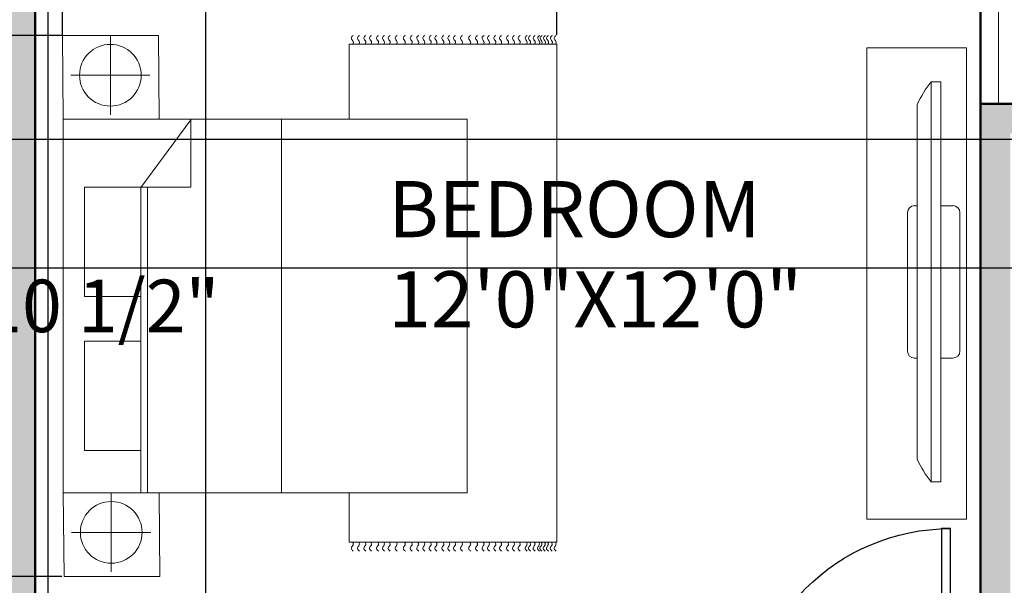
# Model space of a CAD drawing. Units: inches. Extents: x 22042254 to 25404563, y 17568978 to 17626777.
# Tile 40 of 45: x 22179790 to 22179940, y 17626607 to 17626694. Entities that reach past the tile are written whole.
import ezdxf

# ---------------------------------------------------------------- set-up
doc = ezdxf.new("R2010")
doc.units = ezdxf.units.IN
doc.header["$MEASUREMENT"] = 0
for name, color, linetype, lineweight in [('A-ANNO-DIMS', 2, 'Continuous', 18), ('A-AREA-IDEN', 7, 'Continuous', 18), ('A-FLOR-OPEN', 252, 'Continuous', 18), ('A-WALL-PATT', 244, 'Continuous', 13), ('doors', 4, 'Continuous', 25), ('furniture', 8, 'Continuous', 18), ('walls', 252, 'Continuous', 50)]:
    doc.layers.add(name, color=color, linetype=linetype, lineweight=lineweight)
doc.styles.get("Standard").update_dxf_attribs({"font": 'arial.ttf'})
doc.dimstyles.get("Standard").update_dxf_attribs({"dimtxt": 8, "dimasz": 0.18, "dimexe": 0.18, "dimexo": 0.0625, "dimgap": 0.09, "dimtad": 0, "dimtih": 1, "dimtoh": 1, "dimzin": 0, "dimdsep": 46, "dimlunit": 3, "dimtxsty": 'Standard', "dimcen": 0.09, "dimadec": 0, "dimazin": 0, "dimtfac": 1, "dimtofl": 0, "dimtmove": 0, "dimatfit": 3, "dimfxl": 1, "dimtolj": 1, "dimtzin": 0, "dimarcsym": 0})

# ---------------------------------------------------------------- blocks, each defined once
blk = doc.blocks.new('CARPET')
at = {"layer": 'furniture'}
for p, q in [((-51.53, -98.11), (-51.53, -55.12)), ((-51.53, -55.12), (-41.27, -55.12)), ((36, -55.12), (51.55, -55.12)), ((51.55, -55.12), (51.55, -98.11)), ((51.55, -98.11), (-51.53, -98.11))]:
    blk.add_line(p, q, dxfattribs=at)
for points, knots in [([(-53.37, -55.99), (-53.22, -55.8), (-52.9, -55.41), (-52.34, -55.8), (-51.89, -56.08), (-51.65, -55.91), (-51.53, -55.83)], [0, 0, 0, 0, 0.653278, 1.290138, 1.740457, 2.114451, 2.114451, 2.114451, 2.114451]), ([(-53.37, -57.26), (-53.22, -57.07), (-52.9, -56.67), (-52.34, -57.07), (-51.89, -57.35), (-51.65, -57.17), (-51.53, -57.1)], [0, 0, 0, 0, 0.653278, 1.290138, 1.740457, 2.114451, 2.114451, 2.114451, 2.114451]), ([(53.37, -55.99), (53.22, -55.8), (52.9, -55.41), (52.34, -55.8), (51.89, -56.08), (51.65, -55.91), (51.53, -55.83)], [0, 0, 0, 0, 0.653278, 1.290138, 1.740457, 2.114451, 2.114451, 2.114451, 2.114451]), ([(53.37, -57.26), (53.22, -57.07), (52.9, -56.67), (52.34, -57.07), (51.89, -57.35), (51.65, -57.17), (51.53, -57.1)], [0, 0, 0, 0, 0.653278, 1.290138, 1.740457, 2.114451, 2.114451, 2.114451, 2.114451]), ([(-53.37, -58.59), (-53.22, -58.4), (-52.9, -58.01), (-52.34, -58.4), (-51.89, -58.68), (-51.65, -58.5), (-51.53, -58.43)], [0, 0, 0, 0, 0.653278, 1.290138, 1.740457, 2.114451, 2.114451, 2.114451, 2.114451]), ([(53.37, -58.59), (53.22, -58.4), (52.9, -58.01), (52.34, -58.4), (51.89, -58.68), (51.65, -58.5), (51.53, -58.43)], [0, 0, 0, 0, 0.653278, 1.290138, 1.740457, 2.114451, 2.114451, 2.114451, 2.114451]), ([(-53.37, -59.78), (-53.22, -59.58), (-52.9, -59.19), (-52.34, -59.58), (-51.89, -59.86), (-51.65, -59.69), (-51.53, -59.61)], [0, 0, 0, 0, 0.653278, 1.290138, 1.740457, 2.114451, 2.114451, 2.114451, 2.114451]), ([(-53.37, -61.22), (-53.22, -61.02), (-52.9, -60.63), (-52.34, -61.02), (-51.89, -61.3), (-51.65, -61.13), (-51.53, -61.05)], [0, 0, 0, 0, 0.653278, 1.290138, 1.740457, 2.114451, 2.114451, 2.114451, 2.114451]), ([(53.37, -59.78), (53.22, -59.58), (52.9, -59.19), (52.34, -59.58), (51.89, -59.86), (51.65, -59.69), (51.53, -59.61)], [0, 0, 0, 0, 0.653278, 1.290138, 1.740457, 2.114451, 2.114451, 2.114451, 2.114451]), ([(53.37, -61.22), (53.22, -61.02), (52.9, -60.63), (52.34, -61.02), (51.89, -61.3), (51.65, -61.13), (51.53, -61.05)], [0, 0, 0, 0, 0.653278, 1.290138, 1.740457, 2.114451, 2.114451, 2.114451, 2.114451]), ([(-53.37, -62.44), (-53.22, -62.25), (-52.9, -61.86), (-52.34, -62.25), (-51.89, -62.53), (-51.65, -62.36), (-51.53, -62.28)], [0, 0, 0, 0, 0.653278, 1.290138, 1.740457, 2.114451, 2.114451, 2.114451, 2.114451]), ([(-53.37, -63.63), (-53.22, -63.43), (-52.9, -63.04), (-52.34, -63.43), (-51.89, -63.72), (-51.65, -63.54), (-51.53, -63.46)], [0, 0, 0, 0, 0.653278, 1.290138, 1.740457, 2.114451, 2.114451, 2.114451, 2.114451]), ([(53.37, -62.44), (53.22, -62.25), (52.9, -61.86), (52.34, -62.25), (51.89, -62.53), (51.65, -62.36), (51.53, -62.28)], [0, 0, 0, 0, 0.653278, 1.290138, 1.740457, 2.114451, 2.114451, 2.114451, 2.114451]), ([(53.37, -63.63), (53.22, -63.43), (52.9, -63.04), (52.34, -63.43), (51.89, -63.72), (51.65, -63.54), (51.53, -63.46)], [0, 0, 0, 0, 0.653278, 1.290138, 1.740457, 2.114451, 2.114451, 2.114451, 2.114451]), ([(-53.37, -65.07), (-53.22, -64.87), (-52.9, -64.48), (-52.34, -64.87), (-51.89, -65.15), (-51.65, -64.98), (-51.53, -64.9)], [0, 0, 0, 0, 0.653278, 1.290138, 1.740457, 2.114451, 2.114451, 2.114451, 2.114451]), ([(53.37, -65.07), (53.22, -64.87), (52.9, -64.48), (52.34, -64.87), (51.89, -65.15), (51.65, -64.98), (51.53, -64.9)], [0, 0, 0, 0, 0.653278, 1.290138, 1.740457, 2.114451, 2.114451, 2.114451, 2.114451]), ([(-53.37, -66.76), (-53.22, -66.56), (-52.9, -66.17), (-52.34, -66.56), (-51.89, -66.84), (-51.65, -66.67), (-51.53, -66.59)], [0, 0, 0, 0, 0.653278, 1.290138, 1.740457, 2.114451, 2.114451, 2.114451, 2.114451]), ([(53.37, -66.76), (53.22, -66.56), (52.9, -66.17), (52.34, -66.56), (51.89, -66.84), (51.65, -66.67), (51.53, -66.59)], [0, 0, 0, 0, 0.653278, 1.290138, 1.740457, 2.114451, 2.114451, 2.114451, 2.114451]), ([(-53.37, -68.2), (-53.22, -68), (-52.9, -67.61), (-52.34, -68), (-51.89, -68.28), (-51.65, -68.11), (-51.53, -68.03)], [0, 0, 0, 0, 0.653278, 1.290138, 1.740457, 2.114451, 2.114451, 2.114451, 2.114451]), ([(-53.37, -69.53), (-53.22, -69.33), (-52.9, -68.94), (-52.34, -69.33), (-51.89, -69.61), (-51.65, -69.44), (-51.53, -69.36)], [0, 0, 0, 0, 0.653278, 1.290138, 1.740457, 2.114451, 2.114451, 2.114451, 2.114451]), ([(53.37, -68.2), (53.22, -68), (52.9, -67.61), (52.34, -68), (51.89, -68.28), (51.65, -68.11), (51.53, -68.03)], [0, 0, 0, 0, 0.653278, 1.290138, 1.740457, 2.114451, 2.114451, 2.114451, 2.114451]), ([(53.37, -69.53), (53.22, -69.33), (52.9, -68.94), (52.34, -69.33), (51.89, -69.61), (51.65, -69.44), (51.53, -69.36)], [0, 0, 0, 0, 0.653278, 1.290138, 1.740457, 2.114451, 2.114451, 2.114451, 2.114451]), ([(-53.37, -70.79), (-53.22, -70.6), (-52.9, -70.21), (-52.34, -70.6), (-51.89, -70.88), (-51.65, -70.7), (-51.53, -70.63)], [0, 0, 0, 0, 0.653278, 1.290138, 1.740457, 2.114451, 2.114451, 2.114451, 2.114451]), ([(53.37, -70.79), (53.22, -70.6), (52.9, -70.21), (52.34, -70.6), (51.89, -70.88), (51.65, -70.7), (51.53, -70.63)], [0, 0, 0, 0, 0.653278, 1.290138, 1.740457, 2.114451, 2.114451, 2.114451, 2.114451]), ([(-53.37, -72.12), (-53.22, -71.93), (-52.9, -71.54), (-52.34, -71.93), (-51.89, -72.21), (-51.65, -72.04), (-51.53, -71.96)], [0, 0, 0, 0, 0.653278, 1.290138, 1.740457, 2.114451, 2.114451, 2.114451, 2.114451]), ([(-53.37, -73.31), (-53.22, -73.11), (-52.9, -72.72), (-52.34, -73.11), (-51.89, -73.4), (-51.65, -73.22), (-51.53, -73.14)], [0, 0, 0, 0, 0.653278, 1.290138, 1.740457, 2.114451, 2.114451, 2.114451, 2.114451]), ([(53.37, -72.12), (53.22, -71.93), (52.9, -71.54), (52.34, -71.93), (51.89, -72.21), (51.65, -72.04), (51.53, -71.96)], [0, 0, 0, 0, 0.653278, 1.290138, 1.740457, 2.114451, 2.114451, 2.114451, 2.114451]), ([(53.37, -73.31), (53.22, -73.11), (52.9, -72.72), (52.34, -73.11), (51.89, -73.4), (51.65, -73.22), (51.53, -73.14)], [0, 0, 0, 0, 0.653278, 1.290138, 1.740457, 2.114451, 2.114451, 2.114451, 2.114451]), ([(-53.37, -74.75), (-53.22, -74.55), (-52.9, -74.16), (-52.34, -74.55), (-51.89, -74.83), (-51.65, -74.66), (-51.53, -74.58)], [0, 0, 0, 0, 0.653278, 1.290138, 1.740457, 2.114451, 2.114451, 2.114451, 2.114451]), ([(53.37, -74.75), (53.22, -74.55), (52.9, -74.16), (52.34, -74.55), (51.89, -74.83), (51.65, -74.66), (51.53, -74.58)], [0, 0, 0, 0, 0.653278, 1.290138, 1.740457, 2.114451, 2.114451, 2.114451, 2.114451]), ([(-53.37, -75.98), (-53.22, -75.78), (-52.9, -75.39), (-52.34, -75.78), (-51.89, -76.06), (-51.65, -75.89), (-51.53, -75.81)], [0, 0, 0, 0, 0.653278, 1.290138, 1.740457, 2.114451, 2.114451, 2.114451, 2.114451]), ([(-53.37, -77.16), (-53.22, -76.96), (-52.9, -76.57), (-52.34, -76.96), (-51.89, -77.25), (-51.65, -77.07), (-51.53, -76.99)], [0, 0, 0, 0, 0.653278, 1.290138, 1.740457, 2.114451, 2.114451, 2.114451, 2.114451]), ([(53.37, -75.98), (53.22, -75.78), (52.9, -75.39), (52.34, -75.78), (51.89, -76.06), (51.65, -75.89), (51.53, -75.81)], [0, 0, 0, 0, 0.653278, 1.290138, 1.740457, 2.114451, 2.114451, 2.114451, 2.114451]), ([(53.37, -77.16), (53.22, -76.96), (52.9, -76.57), (52.34, -76.96), (51.89, -77.25), (51.65, -77.07), (51.53, -76.99)], [0, 0, 0, 0, 0.653278, 1.290138, 1.740457, 2.114451, 2.114451, 2.114451, 2.114451]), ([(-53.37, -78.6), (-53.22, -78.4), (-52.9, -78.01), (-52.34, -78.4), (-51.89, -78.68), (-51.65, -78.51), (-51.53, -78.43)], [0, 0, 0, 0, 0.653278, 1.290138, 1.740457, 2.114451, 2.114451, 2.114451, 2.114451]), ([(53.37, -78.6), (53.22, -78.4), (52.9, -78.01), (52.34, -78.4), (51.89, -78.68), (51.65, -78.51), (51.53, -78.43)], [0, 0, 0, 0, 0.653278, 1.290138, 1.740457, 2.114451, 2.114451, 2.114451, 2.114451]), ([(-53.37, -80.29), (-53.22, -80.09), (-52.9, -79.7), (-52.34, -80.09), (-51.89, -80.37), (-51.65, -80.2), (-51.53, -80.12)], [0, 0, 0, 0, 0.653278, 1.290138, 1.740457, 2.114451, 2.114451, 2.114451, 2.114451]), ([(-53.37, -81.73), (-53.22, -81.53), (-52.9, -81.14), (-52.34, -81.53), (-51.89, -81.81), (-51.65, -81.64), (-51.53, -81.56)], [0, 0, 0, 0, 0.653278, 1.290138, 1.740457, 2.114451, 2.114451, 2.114451, 2.114451]), ([(53.37, -80.29), (53.22, -80.09), (52.9, -79.7), (52.34, -80.09), (51.89, -80.37), (51.65, -80.2), (51.53, -80.12)], [0, 0, 0, 0, 0.653278, 1.290138, 1.740457, 2.114451, 2.114451, 2.114451, 2.114451]), ([(53.37, -81.73), (53.22, -81.53), (52.9, -81.14), (52.34, -81.53), (51.89, -81.81), (51.65, -81.64), (51.53, -81.56)], [0, 0, 0, 0, 0.653278, 1.290138, 1.740457, 2.114451, 2.114451, 2.114451, 2.114451]), ([(-53.37, -83.06), (-53.22, -82.86), (-52.9, -82.47), (-52.34, -82.86), (-51.89, -83.14), (-51.65, -82.97), (-51.53, -82.89)], [0, 0, 0, 0, 0.653278, 1.290138, 1.740457, 2.114451, 2.114451, 2.114451, 2.114451]), ([(53.37, -83.06), (53.22, -82.86), (52.9, -82.47), (52.34, -82.86), (51.89, -83.14), (51.65, -82.97), (51.53, -82.89)], [0, 0, 0, 0, 0.653278, 1.290138, 1.740457, 2.114451, 2.114451, 2.114451, 2.114451]), ([(-53.37, -84.18), (-53.22, -83.99), (-52.9, -83.6), (-52.34, -83.99), (-51.89, -84.27), (-51.65, -84.09), (-51.53, -84.02)], [0, 0, 0, 0, 0.653278, 1.290138, 1.740457, 2.114451, 2.114451, 2.114451, 2.114451]), ([(-53.37, -85.51), (-53.22, -85.32), (-52.9, -84.93), (-52.34, -85.32), (-51.89, -85.6), (-51.65, -85.42), (-51.53, -85.35)], [0, 0, 0, 0, 0.653278, 1.290138, 1.740457, 2.114451, 2.114451, 2.114451, 2.114451]), ([(53.37, -84.18), (53.22, -83.99), (52.9, -83.6), (52.34, -83.99), (51.89, -84.27), (51.65, -84.09), (51.53, -84.02)], [0, 0, 0, 0, 0.653278, 1.290138, 1.740457, 2.114451, 2.114451, 2.114451, 2.114451]), ([(53.37, -85.51), (53.22, -85.32), (52.9, -84.93), (52.34, -85.32), (51.89, -85.6), (51.65, -85.42), (51.53, -85.35)], [0, 0, 0, 0, 0.653278, 1.290138, 1.740457, 2.114451, 2.114451, 2.114451, 2.114451]), ([(-53.37, -86.7), (-53.22, -86.5), (-52.9, -86.11), (-52.34, -86.5), (-51.89, -86.78), (-51.65, -86.61), (-51.53, -86.53)], [0, 0, 0, 0, 0.653278, 1.290138, 1.740457, 2.114451, 2.114451, 2.114451, 2.114451]), ([(53.37, -86.7), (53.22, -86.5), (52.9, -86.11), (52.34, -86.5), (51.89, -86.78), (51.65, -86.61), (51.53, -86.53)], [0, 0, 0, 0, 0.653278, 1.290138, 1.740457, 2.114451, 2.114451, 2.114451, 2.114451]), ([(-53.37, -88.14), (-53.22, -87.94), (-52.9, -87.55), (-52.34, -87.94), (-51.89, -88.22), (-51.65, -88.05), (-51.53, -87.97)], [0, 0, 0, 0, 0.653278, 1.290138, 1.740457, 2.114451, 2.114451, 2.114451, 2.114451]), ([(-53.37, -89.36), (-53.22, -89.17), (-52.9, -88.78), (-52.34, -89.17), (-51.89, -89.45), (-51.65, -89.28), (-51.53, -89.2)], [0, 0, 0, 0, 0.653278, 1.290138, 1.740457, 2.114451, 2.114451, 2.114451, 2.114451]), ([(53.37, -88.14), (53.22, -87.94), (52.9, -87.55), (52.34, -87.94), (51.89, -88.22), (51.65, -88.05), (51.53, -87.97)], [0, 0, 0, 0, 0.653278, 1.290138, 1.740457, 2.114451, 2.114451, 2.114451, 2.114451]), ([(53.37, -89.36), (53.22, -89.17), (52.9, -88.78), (52.34, -89.17), (51.89, -89.45), (51.65, -89.28), (51.53, -89.2)], [0, 0, 0, 0, 0.653278, 1.290138, 1.740457, 2.114451, 2.114451, 2.114451, 2.114451]), ([(-53.37, -90.55), (-53.22, -90.35), (-52.9, -89.96), (-52.34, -90.35), (-51.89, -90.64), (-51.65, -90.46), (-51.53, -90.38)], [0, 0, 0, 0, 0.653278, 1.290138, 1.740457, 2.114451, 2.114451, 2.114451, 2.114451]), ([(-53.37, -91.99), (-53.22, -91.79), (-52.9, -91.4), (-52.34, -91.79), (-51.89, -92.07), (-51.65, -91.9), (-51.53, -91.82)], [0, 0, 0, 0, 0.653278, 1.290138, 1.740457, 2.114451, 2.114451, 2.114451, 2.114451]), ([(53.37, -90.55), (53.22, -90.35), (52.9, -89.96), (52.34, -90.35), (51.9, -90.63), (51.66, -90.47), (51.55, -90.4)], [0, 0, 0, 0, 0.653278, 1.290138, 1.740457, 2.0926, 2.0926, 2.0926, 2.0926]), ([(53.37, -91.99), (53.22, -91.79), (52.9, -91.4), (52.34, -91.79), (51.9, -92.07), (51.66, -91.91), (51.55, -91.83)], [0, 0, 0, 0, 0.653278, 1.290138, 1.740457, 2.0926, 2.0926, 2.0926, 2.0926]), ([(-53.37, -92.69), (-53.22, -92.48), (-52.9, -92.08), (-52.35, -92.49), (-51.89, -92.77), (-51.65, -92.6), (-51.53, -92.52)], [0, 0, 0, 0, 0.663904, 1.307406, 1.757725, 2.131719, 2.131719, 2.131719, 2.131719]), ([(-53.37, -93.61), (-53.22, -93.42), (-52.9, -93.03), (-52.34, -93.42), (-51.89, -93.7), (-51.65, -93.52), (-51.53, -93.45)], [0, 0, 0, 0, 0.653278, 1.290138, 1.740457, 2.114451, 2.114451, 2.114451, 2.114451]), ([(53.37, -92.69), (53.22, -92.49), (52.9, -92.09), (52.34, -92.49), (51.9, -92.77), (51.66, -92.61), (51.55, -92.53)], [0, 0, 0, 0, 0.656792, 1.295826, 1.746145, 2.098292, 2.098292, 2.098292, 2.098292]), ([(53.37, -93.66), (53.22, -93.46), (52.9, -93.07), (52.34, -93.46), (51.9, -93.74), (51.66, -93.58), (51.55, -93.5)], [0, 0, 0, 0, 0.653278, 1.290138, 1.740457, 2.0926, 2.0926, 2.0926, 2.0926]), ([(-53.37, -94.55), (-53.22, -94.35), (-52.9, -93.96), (-52.34, -94.35), (-51.89, -94.63), (-51.65, -94.46), (-51.53, -94.38)], [0, 0, 0, 0, 0.653278, 1.290138, 1.740457, 2.114451, 2.114451, 2.114451, 2.114451]), ([(-53.37, -95.05), (-53.22, -94.85), (-52.9, -94.46), (-52.34, -94.85), (-51.89, -95.14), (-51.65, -94.96), (-51.53, -94.88)], [0, 0, 0, 0, 0.653278, 1.290138, 1.740457, 2.114451, 2.114451, 2.114451, 2.114451]), ([(-53.37, -95.73), (-53.22, -95.54), (-52.9, -95.15), (-52.34, -95.54), (-51.89, -95.82), (-51.65, -95.65), (-51.53, -95.57)], [0, 0, 0, 0, 0.653278, 1.290138, 1.740457, 2.114451, 2.114451, 2.114451, 2.114451]), ([(53.37, -95.78), (53.22, -95.58), (52.9, -95.19), (52.34, -95.58), (51.89, -95.86), (51.65, -95.69), (51.53, -95.61)], [0, 0, 0, 0, 0.653278, 1.290138, 1.740457, 2.114451, 2.114451, 2.114451, 2.114451]), ([(53.37, -94.59), (53.22, -94.4), (52.9, -94.01), (52.34, -94.4), (51.9, -94.68), (51.66, -94.51), (51.55, -94.44)], [0, 0, 0, 0, 0.653278, 1.290138, 1.740457, 2.0926, 2.0926, 2.0926, 2.0926]), ([(53.37, -95.1), (53.22, -94.9), (52.9, -94.51), (52.34, -94.9), (51.9, -95.18), (51.66, -95.02), (51.55, -94.94)], [0, 0, 0, 0, 0.653278, 1.290138, 1.740457, 2.0926, 2.0926, 2.0926, 2.0926]), ([(-53.37, -96.38), (-53.22, -96.18), (-52.9, -95.79), (-52.34, -96.18), (-51.89, -96.47), (-51.65, -96.29), (-51.53, -96.21)], [0, 0, 0, 0, 0.653278, 1.290138, 1.740457, 2.114451, 2.114451, 2.114451, 2.114451]), ([(-53.37, -97.17), (-53.22, -96.98), (-52.9, -96.59), (-52.34, -96.98), (-51.89, -97.26), (-51.65, -97.08), (-51.53, -97.01)], [0, 0, 0, 0, 0.653278, 1.290138, 1.740457, 2.114451, 2.114451, 2.114451, 2.114451]), ([(-53.37, -97.99), (-53.22, -97.79), (-52.9, -97.4), (-52.34, -97.79), (-51.89, -98.08), (-51.65, -97.9), (-51.53, -97.82)], [0, 0, 0, 0, 0.653278, 1.290138, 1.740457, 2.114451, 2.114451, 2.114451, 2.114451]), ([(53.37, -96.43), (53.22, -96.23), (52.9, -95.84), (52.34, -96.23), (51.89, -96.51), (51.65, -96.34), (51.53, -96.26)], [0, 0, 0, 0, 0.653278, 1.290138, 1.740457, 2.114451, 2.114451, 2.114451, 2.114451]), ([(53.37, -97.22), (53.22, -97.02), (52.9, -96.63), (52.34, -97.02), (51.89, -97.3), (51.65, -97.13), (51.53, -97.05)], [0, 0, 0, 0, 0.653278, 1.290138, 1.740457, 2.114451, 2.114451, 2.114451, 2.114451]), ([(53.37, -97.99), (53.22, -97.79), (52.9, -97.4), (52.34, -97.79), (51.89, -98.08), (51.65, -97.9), (51.53, -97.82)], [0, 0, 0, 0, 0.653278, 1.290138, 1.740457, 2.114451, 2.114451, 2.114451, 2.114451])]:
    blk.add_open_spline(points, degree=3, knots=knots, dxfattribs=at)
blk = doc.blocks.new('A$C58D270C6')
at = {"layer": 'furniture'}
for p, q in [((9.09, 124.13), (9.09, 108.87)), ((1.46, 116.5), (16.73, 116.5)), ((14.97, 94.84), (24.62, 107.92)), ((24.62, 94.93), (24.62, 107.92)), ((42.08, 108), (42.08, 36)), ((14.97, 94.93), (24.62, 94.93)), ((16.22, 94.93), (16.22, 36)), ((14.97, 94.84), (14.97, 36)), ((9.25, 36), (9.25, 20.74)), ((1.62, 28.37), (16.88, 28.37))]:
    blk.add_line(p, q, dxfattribs=at)
for points in [[(18.5, 108), (18.34, 124.13), (-0.16, 124.13), (0, 108)], [(0, 108), (77.91, 108), (77.91, 36), (0, 36)], [(4.09, 94.93), (14.97, 94.93), (14.97, 73.83), (4.09, 73.83)], [(4.09, 65.23), (14.97, 65.23), (14.97, 44.13), (4.09, 44.13)], [(18.65, 19.87), (18.5, 36), (0, 36), (0.16, 19.87)]]:
    blk.add_lwpolyline(points, close=True, dxfattribs=at)
for centre in [(9.09, 116.5), (9.25, 28.37)]:
    blk.add_circle(centre, 5.95, dxfattribs=at)
at = {"layer": 'furniture', "xscale": 0.9312884925094044, "yscale": 0.9312884925094044, "zscale": 0.9312884925094044, "rotation": 90}
blk.add_blockref('CARPET', (3.79, 74.47), dxfattribs=at)
blk = doc.blocks.new('*U24')
for p, q in [((0, 0), (0, -6)), ((40, 0), (40, -6))]:
    blk.add_line(p, q)
blk.add_lwpolyline([(0, 0), (0, 40), (1.75, 40), (1.75, 0)], close=True)
blk.add_arc((0, 0), 40, 0, 90)
blk = doc.blocks.new('PLASMA-LARGE')
at = {"layer": 'furniture'}
for p, q in [((-7.26, 0), (7.26, 0)), ((-18.61, -1), (18.61, -1)), ((-8, -1), (-8, -0.74)), ((8, -1), (8, -0.74)), ((-21, -2.5), (21, -2.5)), ((-21, -2.5), (-21, -3.5)), ((21, -2.5), (21, -3.5)), ((-21, -3.5), (21, -3.5)), ((-8, -3.5), (-8, -4.76)), ((8, -3.5), (8, -4.76)), ((-7.26, -5.5), (7.26, -5.5))]:
    blk.add_line(p, q, dxfattribs=at)
for centre, radius, start, end in [((-7.26, -0.74), 0.744, 90, 180), ((7.26, -0.74), 0.744, 0, 90), ((-13.97, -11.05), 11.07, 114.7602, 129.4175), ((13.97, -11.05), 11.07, 50.5825, 65.2398), ((-7.26, -4.76), 0.744, 180, 270), ((7.26, -4.76), 0.744, 270, 0)]:
    blk.add_arc(centre, radius, start, end, dxfattribs=at)
blk = doc.blocks.new('TV-CONSOLE')
for p, q in [((8.99, 35.63), (-6.22, 35.63)), ((-6.22, 35.63), (-6.22, -36.14)), ((8.99, -36.14), (8.99, 35.63)), ((-6.22, -36.14), (8.99, -36.14))]:
    blk.add_line(p, q)
at = {"xscale": 1.450199298177205, "yscale": 1.450199298177205, "zscale": 1.450199298177205, "rotation": 90}
blk.add_blockref('PLASMA-LARGE', (0, 0), dxfattribs=at)
blk = doc.blocks.new('*D30')
at = {"layer": 'A-ANNO-DIMS', "color": 0, "lineweight": -2, "transparency": 16777216}
for p, q in [((22179796.84, 17626691.22), (22179784.37, 17626691.22)), ((22179784.55, 17626691.04), (22179784.55, 17626654.25)), ((22179784.55, 17626609.02), (22179784.55, 17626645.8)), ((22179796.84, 17626608.84), (22179784.37, 17626608.84))]:
    blk.add_line(p, q, dxfattribs=at)
at = {"layer": 'A-ANNO-DIMS', "color": 0, "transparency": 16777216}
for points in [[(22179784.52, 17626691.04), (22179784.58, 17626691.04), (22179784.55, 17626691.22)], [(22179784.52, 17626609.02), (22179784.58, 17626609.02), (22179784.55, 17626608.84)]]:
    blk.add_solid(points, dxfattribs=at)
at = {"layer": 'Defpoints', "color": 0, "transparency": 16777216}
for p in [(22179784.55, 17626691.22), (22179796.91, 17626691.22), (22179796.91, 17626608.84)]:
    blk.add_point(p, dxfattribs=at)
at = {"layer": 'A-ANNO-DIMS', "color": 0, "transparency": 16777216, "insert": (22179784.55, 17626650.03), "char_height": 8, "attachment_point": 5}
blk.add_mtext('\\A1;BED 6\'-10 1/2"', dxfattribs=at)
blk = doc.blocks.new('*D31')
at = {"layer": 'A-ANNO-DIMS', "color": 0, "lineweight": -2, "transparency": 16777216}
for p, q in [((22179796.91, 17626691.28), (22179796.91, 17626703.76)), ((22179797.09, 17626703.58), (22179814.48, 17626703.58)), ((22179872.01, 17626703.58), (22179854.61, 17626703.58)), ((22179872.19, 17626691.28), (22179872.19, 17626703.76))]:
    blk.add_line(p, q, dxfattribs=at)
at = {"layer": 'A-ANNO-DIMS', "color": 0, "transparency": 16777216}
for points in [[(22179797.09, 17626703.61), (22179797.09, 17626703.55), (22179796.91, 17626703.58)], [(22179872.01, 17626703.61), (22179872.01, 17626703.55), (22179872.19, 17626703.58)]]:
    blk.add_solid(points, dxfattribs=at)
at = {"layer": 'Defpoints', "color": 0, "transparency": 16777216}
for p in [(22179872.19, 17626703.58), (22179796.91, 17626691.22), (22179872.19, 17626691.22)]:
    blk.add_point(p, dxfattribs=at)
at = {"layer": 'A-ANNO-DIMS', "color": 0, "transparency": 16777216, "insert": (22179834.55, 17626703.58), "char_height": 8, "attachment_point": 5}
blk.add_mtext('\\A1;6\'-3 1/2"', dxfattribs=at)
blk = doc.blocks.new('*D46')
at = {"layer": 'A-ANNO-DIMS', "color": 0, "lineweight": -2, "transparency": 16777216}
for p, q in [((22179959.69, 17626609.47), (22179963.21, 17626609.47)), ((22179963.03, 17626609.29), (22179963.03, 17626602.36)), ((22179963.03, 17626586.98), (22179963.03, 17626593.91)), ((22179959.69, 17626586.8), (22179963.21, 17626586.8))]:
    blk.add_line(p, q, dxfattribs=at)
at = {"layer": 'A-ANNO-DIMS', "color": 0, "transparency": 16777216}
for points in [[(22179963, 17626609.29), (22179963.06, 17626609.29), (22179963.03, 17626609.47)], [(22179963, 17626586.98), (22179963.06, 17626586.98), (22179963.03, 17626586.8)]]:
    blk.add_solid(points, dxfattribs=at)
at = {"layer": 'Defpoints', "color": 0, "transparency": 16777216}
for p in [(22179959.63, 17626609.47), (22179963.03, 17626609.47), (22179959.63, 17626586.8)]:
    blk.add_point(p, dxfattribs=at)
at = {"layer": 'A-ANNO-DIMS', "color": 0, "transparency": 16777216, "insert": (22179963.03, 17626598.14), "char_height": 8, "attachment_point": 5}
blk.add_mtext('\\A1;BASIN 1\'-10 1/2" TYP.', dxfattribs=at)
blk = doc.blocks.new('*D60')
at = {"layer": 'A-ANNO-DIMS', "color": 0, "lineweight": -2, "transparency": 16777216}
for p, q in [((22179794.73, 17626555.5), (22179794.73, 17626772.16)), ((22179794.91, 17626771.98), (22179795.94, 17626771.98)), ((22179818.55, 17626771.98), (22179817.52, 17626771.98)), ((22179818.73, 17626560), (22179818.73, 17626772.16))]:
    blk.add_line(p, q, dxfattribs=at)
at = {"layer": 'A-ANNO-DIMS', "color": 0, "transparency": 16777216}
for points in [[(22179794.91, 17626772.01), (22179794.91, 17626771.95), (22179794.73, 17626771.98)], [(22179818.55, 17626772.01), (22179818.55, 17626771.95), (22179818.73, 17626771.98)]]:
    blk.add_solid(points, dxfattribs=at)
at = {"layer": 'Defpoints', "color": 0, "transparency": 16777216}
for p in [(22179818.73, 17626771.98), (22179818.73, 17626559.94), (22179794.73, 17626555.44)]:
    blk.add_point(p, dxfattribs=at)
at = {"layer": 'A-ANNO-DIMS', "color": 0, "transparency": 16777216, "insert": (22179806.73, 17626771.98), "char_height": 8, "attachment_point": 5}
blk.add_mtext('\\A1;2\'-0"', dxfattribs=at)
blk = doc.blocks.new('*D62')
at = {"layer": 'A-ANNO-DIMS', "color": 0, "lineweight": -2, "transparency": 16777216}
for p, q in [((22179965.84, 17626675.39), (22179727.35, 17626675.39)), ((22179727.53, 17626675.21), (22179727.53, 17626669.81)), ((22179727.53, 17626655.96), (22179727.53, 17626661.36)), ((22179962.16, 17626655.78), (22179727.35, 17626655.78))]:
    blk.add_line(p, q, dxfattribs=at)
at = {"layer": 'A-ANNO-DIMS', "color": 0, "transparency": 16777216}
for points in [[(22179727.5, 17626675.21), (22179727.56, 17626675.21), (22179727.53, 17626675.39)], [(22179727.5, 17626655.96), (22179727.56, 17626655.96), (22179727.53, 17626655.78)]]:
    blk.add_solid(points, dxfattribs=at)
at = {"layer": 'Defpoints', "color": 0, "transparency": 16777216}
for p in [(22179965.9, 17626675.39), (22179727.53, 17626655.78), (22179962.22, 17626655.78)]:
    blk.add_point(p, dxfattribs=at)
at = {"layer": 'A-ANNO-DIMS', "color": 0, "transparency": 16777216, "insert": (22179727.53, 17626665.59), "char_height": 8, "attachment_point": 5}
blk.add_mtext('\\A1;1\'-7 1/2"', dxfattribs=at)

msp = doc.modelspace()

# ---------------------------------------------------------------- hatches: boundary and pattern name
at = {"layer": 'A-WALL-PATT'}
h = msp.add_hatch(color=256, dxfattribs=at)
h.dxf.hatch_style = 1
h.paths.add_polyline_path([(22179792.734, 17626580.28), (22179888.734, 17626580.28), (22179888.734, 17626559.623), (22179893.234, 17626559.623), (22179893.234, 17626580.28), (22179900.438, 17626580.28), (22179900.438, 17626584.78), (22179792.734, 17626584.78), (22179792.734, 17626728.78), (22180134.734, 17626728.78), (22180134.734, 17626584.78), (22180035.602, 17626584.78), (22180004.432, 17626584.78), (22180001.734, 17626584.78), (22180001.734, 17626580.28), (22180134.734, 17626580.28), (22180134.734, 17626404.28), (22180064.487, 17626404.28), (22180064.487, 17626399.78), (22180134.734, 17626399.78), (22180134.734, 17626197.78), (22180143.734, 17626197.78), (22180143.734, 17626737.78), (22179783.734, 17626737.78), (22179783.734, 17626197.78), (22179792.734, 17626197.78), (22179792.734, 17626394.78), (22179936.734, 17626394.78), (22179936.734, 17626383.208), (22179941.234, 17626383.208), (22179941.234, 17626532.28), (22179927.066, 17626532.28), (22179927.066, 17626527.78), (22179928.072, 17626527.78), (22179936.734, 17626527.78), (22179936.734, 17626403.78), (22179792.734, 17626403.78), (22179792.734, 17626527.78), (22179905.094, 17626527.78), (22179905.094, 17626532.28), (22179792.734, 17626532.28)])
h = msp.add_hatch(color=256, dxfattribs=at)
h.dxf.hatch_style = 1
h.paths.add_polyline_path([(22179941.234, 17626676.28), (22179997.234, 17626676.28), (22179997.234, 17626614.838), (22180001.734, 17626614.838), (22180001.734, 17626680.78), (22179936.734, 17626680.78), (22179936.734, 17626617.551), (22179936.734, 17626580.28), (22179941.234, 17626580.28), (22180001.734, 17626580.28), (22180001.734, 17626591.815), (22179997.234, 17626591.815), (22179997.234, 17626584.78), (22179941.234, 17626584.78)])

# ---------------------------------------------------------------- linework, layer by layer
at = {"layer": 'A-FLOR-OPEN'}
msp.add_line((22179939.449, 17626680.78), (22179939.449, 17626728.78), dxfattribs=at)
at = {"layer": 'walls'}
for p, q in [((22179792.734, 17626584.78), (22179792.734, 17626728.78)), ((22179936.734, 17626580.28), (22179936.734, 17626728.78)), ((22179936.734, 17626680.78), (22180001.734, 17626680.78))]:
    msp.add_line(p, q, dxfattribs=at)

# ---------------------------------------------------------------- block references
at = {"layer": 'doors', "xscale": -0.7792671805443983, "yscale": 0.7792671805443983, "zscale": 0.7792671805443983}
msp.add_blockref('*U24', (22179932.13, 17626584.955), dxfattribs=at)
at = {"layer": 'furniture', "xscale": 0.7897983012973059, "yscale": 0.7897983012973059, "zscale": 0.7897983012973059}
msp.add_blockref('A$C58D270C6', (22179797.03, 17626593.143), dxfattribs=at)
at = {"layer": 'furniture'}
msp.add_blockref('TV-CONSOLE', (22179925.602, 17626653.686), dxfattribs=at)

# ---------------------------------------------------------------- texts
at = {"layer": 'A-AREA-IDEN'}
for s, height, p in [('BEDROOM', 8.5453, (22179846.543, 17626660.494)), ('12\'0"X12\'0"', 8.54529, (22179846.543, 17626646.767))]:
    msp.add_text(s, height=height, dxfattribs=at).set_placement(p)

# ---------------------------------------------------------------- dimensions: what is measured, and where the dimension line sits
at = {"layer": 'A-ANNO-DIMS'}
for base, p1, p2, picture, middle in [((22179818.734, 17626771.98), (22179794.734, 17626555.436), (22179818.734, 17626559.936), '*D60', (22179806.734, 17626771.98)), ((22179872.186, 17626703.578), (22179796.907, 17626691.22), (22179872.186, 17626691.22), '*D31', (22179834.546, 17626703.578))]:
    dim = msp.add_linear_dim(base=base, p1=p1, p2=p2, dimstyle='Standard', override={"dimdec": 1, "dimlfac": 1, "dimrnd": 0, "dimzin": 1, "dimdsep": 46, "dimlunit": 4, "dimfrac": 2}, dxfattribs=at)
    dim.commit()
    dim.dimension.update_dxf_attribs({"geometry": picture, "text_midpoint": middle})
for base, p1, p2, text, picture, middle in [((22179784.549, 17626691.22), (22179796.907, 17626608.836), (22179796.907, 17626691.22), 'BED <>', '*D30', (22179784.549, 17626650.028)), ((22179963.03, 17626609.475), (22179959.629, 17626586.798), (22179959.629, 17626609.475), 'BASIN <> TYP.', '*D46', (22179963.03, 17626598.136))]:
    dim = msp.add_linear_dim(base=base, p1=p1, p2=p2, angle=90, text=text, dimstyle='Standard', override={"dimdec": 1, "dimlfac": 1, "dimrnd": 0, "dimzin": 1, "dimdsep": 46, "dimlunit": 4, "dimfrac": 2}, dxfattribs=at)
    dim.commit()
    dim.dimension.update_dxf_attribs({"geometry": picture, "text_midpoint": middle})
dim = msp.add_linear_dim(base=(22179727.534, 17626655.782), p1=(22179965.901, 17626675.394), p2=(22179962.224, 17626655.782), angle=90, dimstyle='Standard', override={"dimdec": 1, "dimlfac": 1, "dimrnd": 0, "dimzin": 1, "dimdsep": 46, "dimlunit": 4, "dimfrac": 2}, dxfattribs=at)
dim.commit()
dim.dimension.update_dxf_attribs({"geometry": '*D62', "text_midpoint": (22179727.534, 17626665.588)})

doc.saveas('drawing.dxf')
